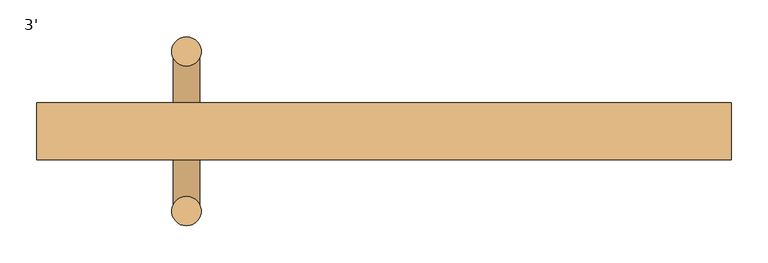
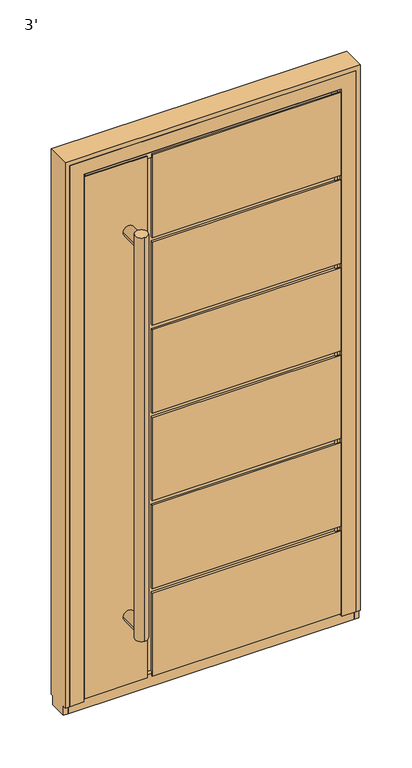
"""IFC4 building model written with IfcOpenShell, lengths in millimetres: door geometry, 3'."""

from ifc_helpers import new_model, si_unit, point, frame, frame_2d, origin, place, context, project, spatial, circle_curve, trimmed, segment, composite_curve, outline, extrude, faceted_brep, source, transform, mapped, element, save


def door_3_44036f4b(model_context):
    return source(origin(), model_context, "Body", "SolidModel", [
        extrude(outline(composite_curve([segment(trimmed(circle_curve(frame_2d((-268.65, 90.8003001)), 20.0), [point((-268.65, 70.8003001))], [point((-268.65, 110.8003001))], False, "CARTESIAN"), True, "CONTINUOUS"), segment(trimmed(circle_curve(frame_2d((-268.65, 90.8003001)), 20.0), [point((-268.65, 110.8003001))], [point((-268.65, 70.8003001))], False, "CARTESIAN"), True, "CONTINUOUS")], self_intersect=False)), frame((0.0, 0.0, 210.0000003), z_axis=(0.0, 0.0, 1.0), x_axis=(1.0, 0.0, 0.0)), (0.0, 0.0, 1.0), 1363.8),
        extrude(outline(composite_curve([segment(trimmed(circle_curve(frame_2d((-268.65, -126.2003001)), 20.0), [point((-268.65, -146.2003001))], [point((-268.65, -106.2003001))], False, "CARTESIAN"), True, "CONTINUOUS"), segment(trimmed(circle_curve(frame_2d((-268.65, -126.2003001)), 20.0), [point((-268.65, -106.2003001))], [point((-268.65, -146.2003001))], False, "CARTESIAN"), True, "CONTINUOUS")], self_intersect=False)), frame((0.0, 0.0, 210.0000003), z_axis=(0.0, 0.0, 1.0), x_axis=(1.0, 0.0, 0.0)), (0.0, 0.0, 1.0), 1363.8),
        extrude(outline(composite_curve([segment(trimmed(circle_curve(frame_2d((241.9000003, -268.65)), 18.0), [point((241.9000003, -286.65))], [point((241.9000003, -250.65))], False, "CARTESIAN"), True, "CONTINUOUS"), segment(trimmed(circle_curve(frame_2d((241.9000003, -268.65)), 18.0), [point((241.9000003, -250.65))], [point((241.9000003, -286.65))], False, "CARTESIAN"), True, "CONTINUOUS")], self_intersect=False)), frame((0.0, -126.2, 0.0), z_axis=(0.0, 1.0, 0.0), x_axis=(0.0, 0.0, 1.0)), (0.0, 0.0, 1.0), 217.0),
        extrude(outline(composite_curve([segment(trimmed(circle_curve(frame_2d((1541.9000003, -268.65)), 18.0), [point((1541.9000003, -286.65))], [point((1541.9000003, -250.65))], False, "CARTESIAN"), True, "CONTINUOUS"), segment(trimmed(circle_curve(frame_2d((1541.9000003, -268.65)), 18.0), [point((1541.9000003, -250.65))], [point((1541.9000003, -286.65))], False, "CARTESIAN"), True, "CONTINUOUS")], self_intersect=False)), frame((0.0, -126.2, 0.0), z_axis=(0.0, 1.0, 0.0), x_axis=(0.0, 0.0, 1.0)), (0.0, 0.0, 1.0), 217.0),
        faceted_brep([(-193.65, 13.8, 306.466667), (383.65, 13.8, 306.466667), (383.65, 13.8, 291.466667), (-193.65, 13.8, 291.466667), (-193.65, 13.8, 35.0), (-208.65, 13.8, 35.0), (-208.65, 13.8, 1748.8000003), (-193.65, 13.8, 1748.8000003), (-193.65, 13.8, 1492.3333337), (383.65, 13.8, 1492.3333337), (383.65, 13.8, 1477.3333337), (-193.65, 13.8, 1477.3333337), (-193.65, 13.8, 1195.866667), (383.65, 13.8, 1195.866667), (383.65, 13.8, 1180.866667), (-193.65, 13.8, 1180.866667), (-193.65, 13.8, 899.4000004), (383.65, 13.8, 899.4000004), (383.65, 13.8, 884.4000004), (-193.65, 13.8, 884.4000004), (-193.65, 13.8, 602.9333337), (383.65, 13.8, 602.9333337), (383.65, 13.8, 587.9333337), (-193.65, 13.8, 587.9333337), (-193.65, 20.8, 587.9333337), (-193.65, 20.8, 306.466667), (383.65, 20.8, 587.9333337), (383.65, 11.7997698, 1748.8000003), (383.65, 11.7997698, 35.0), (383.65, 18.8020472, 35.0), (383.65, 18.8020472, 24.0), (383.65, 20.8, 24.0), (383.65, 20.8, 291.466667), (383.65, 20.8, 306.466667), (383.65, 20.8, 602.9333337), (383.65, 20.8, 884.4000004), (383.65, 20.8, 899.4000004), (383.65, 20.8, 1180.866667), (383.65, 20.8, 1195.866667), (383.65, 20.8, 1477.3333337), (383.65, 20.8, 1492.3333337), (383.65, 20.8, 1748.8000003), (-193.65, 20.8, 602.9333337), (-193.65, 20.8, 884.4000004), (-193.65, 20.8, 899.4000004), (-193.65, 20.8, 1180.866667), (-208.65, 18.8020472, 35.0), (-208.65, 18.8020472, 24.0), (-208.65, 20.8, 24.0), (-208.65, 20.8, 1748.8000003), (-383.65, 11.7997698, 35.0), (-383.65, 18.8020472, 35.0), (-193.65, 18.8020472, 35.0), (-193.65, 20.8, 291.466667), (-193.65, 20.8, 24.0), (-193.65, 18.8020472, 24.0), (-383.65, 18.8020472, 24.0), (-383.65, 20.8, 24.0), (-383.65, 20.8, 1748.8000003), (-193.65, 20.8, 1195.866667), (-193.65, 20.8, 1477.3333337), (-193.65, 20.8, 1492.3333337), (-193.65, 20.8, 1748.8000003), (408.65, -56.2, 10.0000003), (-193.65, -56.2, 10.0000003), (-193.65, -53.2, 10.0000003), (408.65, -53.2, 10.0000003), (-408.65, -53.2, 10.0000003), (-208.65, -53.2, 10.0000003), (-208.65, -56.2, 10.0000003), (-408.65, -56.2, 10.0000003), (408.65, -56.2, 306.466667), (408.65, -53.2, 306.466667), (408.65, -53.2, 587.9333337), (408.65, -56.2, 587.9333337), (408.65, -56.2, 899.4000004), (408.65, -53.2, 899.4000004), (408.65, -53.2, 1180.866667), (408.65, -56.2, 1180.866667), (408.65, -56.2, 602.9333337), (408.65, -53.2, 602.9333337), (408.65, -53.2, 884.4000004), (408.65, -56.2, 884.4000004), (408.65, -56.2, 1195.866667), (408.65, -53.2, 1195.866667), (408.65, -53.2, 1477.3333337), (408.65, -56.2, 1477.3333337), (408.65, -56.2, 1773.8000003), (408.65, -56.2, 1492.3333337), (408.65, -53.2, 1492.3333337), (408.65, -53.2, 1773.8000003), (408.65, -53.2, 291.466667), (408.65, -56.2, 291.466667), (-193.65, -53.2, 25.5), (393.15, -53.2, 25.5), (393.15, -53.2, 291.466667), (393.15, -53.2, 306.466667), (393.15, -53.2, 587.9333337), (393.15, -53.2, 899.4000004), (393.15, -53.2, 1180.866667), (393.15, -53.2, 602.9333337), (393.15, -53.2, 884.4000004), (-393.15, -53.2, 25.5), (-208.65, -53.2, 25.5), (-408.65, -53.2, 1773.8000003), (-208.65, -53.2, 1773.8000003), (-208.65, -53.2, 1758.3000003), (-393.15, -53.2, 1758.3000003), (393.15, -53.2, 1195.866667), (393.15, -53.2, 1477.3333337), (393.15, -53.2, 1492.3333337), (393.15, -53.2, 1758.3000003), (-193.65, -53.2, 1758.3000003), (-193.65, -53.2, 1773.8000003), (-193.65, -49.2, 291.466667), (-193.65, -49.2, 25.5), (-193.65, -56.2, 291.466667), (-208.65, -56.2, 1773.8000003), (-408.65, -56.2, 1773.8000003), (-193.65, -56.2, 587.9333337), (-193.65, -56.2, 306.466667), (-193.65, -56.2, 1180.866667), (-193.65, -56.2, 899.4000004), (-193.65, -56.2, 884.4000004), (-193.65, -56.2, 602.9333337), (-193.65, -56.2, 1477.3333337), (-193.65, -56.2, 1195.866667), (-193.65, -56.2, 1773.8000003), (-193.65, -56.2, 1492.3333337), (-208.65, -49.2, 1758.3000003), (-208.65, -49.2, 25.5), (-383.65, 11.7997698, 1748.8000003), (393.15, 11.7997698, 1758.3000003), (393.15, 11.7997698, 25.5), (-393.15, 11.7997698, 25.5), (-393.15, 11.7997698, 1758.3000003), (393.15, -49.2, 1492.3333337), (393.15, -49.2, 1477.3333337), (393.15, -49.2, 1195.866667), (393.15, -49.2, 1180.866667), (393.15, -49.2, 899.4000004), (393.15, -49.2, 884.4000004), (393.15, -49.2, 602.9333337), (393.15, -49.2, 587.9333337), (393.15, -49.2, 306.466667), (393.15, -49.2, 291.466667), (-193.65, -49.2, 1477.3333337), (-193.65, -49.2, 1492.3333337), (-193.65, -49.2, 1758.3000003), (-193.65, -49.2, 306.466667), (-193.65, -49.2, 587.9333337), (-193.65, -49.2, 602.9333337), (-193.65, -49.2, 884.4000004), (-193.65, -49.2, 899.4000004), (-193.65, -49.2, 1180.866667), (-193.65, -49.2, 1195.866667)], [[[0, 1, 2, 3, 4, 5, 6, 7, 8, 9, 10, 11, 12, 13, 14, 15, 16, 17, 18, 19, 20, 21, 22, 23]], [[23, 24, 25, 0]], [[23, 22, 26, 24]], [[27, 28, 29, 30, 31, 32, 2, 1, 33, 26, 22, 21, 34, 35, 18, 17, 36, 37, 14, 13, 38, 39, 10, 9, 40, 41]], [[42, 34, 21, 20]], [[19, 43, 42, 20]], [[19, 18, 35, 43]], [[44, 36, 17, 16]], [[15, 45, 44, 16]], [[5, 46, 47, 48, 49, 6]], [[28, 50, 51, 46, 5, 4, 52, 29]], [[53, 54, 55, 52, 4, 3]], [[3, 2, 32, 53]], [[25, 33, 1, 0]], [[29, 52, 55, 30]], [[56, 47, 46, 51]], [[30, 55, 54, 31]], [[57, 48, 47, 56]], [[36, 44, 45, 37]], [[34, 42, 43, 35]], [[33, 25, 24, 26]], [[54, 53, 32, 31]], [[58, 49, 48, 57]], [[38, 59, 60, 39]], [[41, 40, 61, 62]], [[63, 64, 65, 66]], [[67, 68, 69, 70]], [[71, 72, 73, 74]], [[75, 76, 77, 78]], [[79, 80, 81, 82]], [[83, 84, 85, 86]], [[87, 88, 89, 90]], [[66, 91, 92, 63]], [[65, 93, 94, 95, 91, 66]], [[72, 96, 97, 73]], [[76, 98, 99, 77]], [[80, 100, 101, 81]], [[102, 103, 68, 67, 104, 105, 106, 107]], [[84, 108, 109, 85]], [[90, 89, 110, 111, 112, 113]], [[114, 115, 93, 65, 64, 116]], [[70, 69, 117, 118]], [[63, 92, 116, 64]], [[74, 119, 120, 71]], [[78, 121, 122, 75]], [[82, 123, 124, 79]], [[86, 125, 126, 83]], [[87, 127, 128, 88]], [[70, 118, 104, 67]], [[129, 106, 105, 117, 69, 68, 103, 130]], [[58, 57, 56, 51, 50, 131]], [[132, 133, 134, 135], [131, 50, 28, 27]], [[111, 110, 136, 137, 109, 108, 138, 139, 99, 98, 140, 141, 101, 100, 142, 143, 97, 96, 144, 145, 95, 94, 133, 132]], [[94, 93, 115, 130, 103, 102, 134, 133]], [[135, 134, 102, 107]], [[146, 137, 136, 147, 148, 129, 130, 115, 114, 145, 144, 149, 150, 143, 142, 151, 152, 141, 140, 153, 154, 139, 138, 155]], [[153, 122, 121, 154]], [[153, 140, 98, 76, 75, 122]], [[123, 82, 81, 101, 141, 152]], [[151, 124, 123, 152]], [[151, 142, 100, 80, 79, 124]], [[119, 74, 73, 97, 143, 150]], [[149, 120, 119, 150]], [[149, 144, 96, 72, 71, 120]], [[116, 92, 91, 95, 145, 114]], [[15, 14, 37, 45]], [[59, 38, 13, 12]], [[11, 60, 59, 12]], [[11, 10, 39, 60]], [[61, 40, 9, 8]], [[8, 7, 62, 61]], [[125, 86, 85, 109, 137, 146]], [[128, 127, 113, 112, 148, 147]], [[121, 78, 77, 99, 139, 154]], [[155, 138, 108, 84, 83, 126]], [[155, 126, 125, 146]], [[147, 136, 110, 89, 88, 128]], [[90, 113, 127, 87]], [[118, 117, 105, 104]], [[132, 135, 107, 106, 129, 148, 112, 111]], [[27, 41, 62, 7, 6, 49, 58, 131]]]),
        faceted_brep([(-457.2, -56.2, 0.0), (-457.2, -47.1997571, 0.0), (-412.7, -47.1997571, 0.0), (-412.7, -56.2, 0.0), (-403.2, 16.2999958, 0.0), (-403.2, 11.8, 0.0), (-457.2, 11.8, 0.0), (-457.2, 20.8, 0.0), (-387.7, 20.8, 0.0), (-387.7, 16.2999958, 0.0), (457.2, 20.8, 0.0), (457.2, 11.8, 0.0), (403.2, 11.8, 0.0), (403.2, 16.2999958, 0.0), (387.7, 16.2999958, 0.0), (387.7, 20.8, 0.0), (412.7, -47.1997571, 0.0), (457.2, -47.1997571, 0.0), (457.2, -56.2, 0.0), (412.7, -56.2, 0.0), (-457.2, 11.8, -30.0), (-457.2, -47.1997571, -30.0), (-457.2, -56.2, 1828.8), (-457.2, 20.8, 1828.8), (-412.7, -56.2, 1784.3), (412.7, -56.2, 1784.3), (457.2, -56.2, 1828.8), (457.2, 20.8, 1828.8), (457.2, -47.1997571, -30.0), (457.2, 11.8, -30.0), (387.7, 20.8, 1759.3), (-387.7, 20.8, 1759.3), (-403.2, -47.2, 1774.8), (-403.2, -47.2, 14.5), (-403.2, 11.8, 14.5), (-403.2, 16.2999958, 1774.8), (403.2, 16.2999958, 1774.8), (403.2, -47.2, 1774.8), (403.2, 11.8, 14.5), (403.2, -47.2, 14.5), (-412.7, -47.2, 1784.3), (412.7, -47.2, 1784.3), (-387.7, 16.2999958, 1759.3), (387.7, 16.2999958, 1759.3)], [[[0, 1, 2, 3]], [[4, 5, 6, 7, 8, 9]], [[10, 11, 12, 13, 14, 15]], [[16, 17, 18, 19]], [[7, 6, 20, 21, 1, 0, 22, 23]], [[3, 24, 25, 19, 18, 26, 22, 0]], [[22, 26, 27, 23]], [[18, 17, 28, 29, 11, 10, 27, 26]], [[7, 23, 27, 10, 15, 30, 31, 8]], [[32, 33, 34, 5, 4, 35]], [[35, 36, 37, 32]], [[36, 13, 12, 38, 39, 37]], [[40, 24, 3, 2]], [[16, 41, 40, 2, 1, 21, 28, 17], [37, 39, 33, 32]], [[9, 42, 43, 14, 13, 36, 35, 4]], [[8, 31, 42, 9]], [[24, 40, 41, 25]], [[30, 43, 42, 31]], [[19, 25, 41, 16]], [[14, 43, 30, 15]], [[20, 6, 5, 34, 38, 12, 11, 29]], [[39, 38, 34, 33]], [[20, 29, 28, 21]]]),
        faceted_brep([(-457.2, -47.2, -30.0), (-472.2, -47.2, -30.0), (-472.2, 11.8, -30.0), (-457.2, 11.8, -30.0), (-457.2, -56.2, 1828.8), (-457.2, -56.2, 0.0), (-457.2, -47.2, 0.0), (-457.2, 11.8, 0.0), (-457.2, 20.8, 0.0), (-457.2, 20.8, 1828.8), (-472.2, 11.8, 0.0), (472.2, 11.8, 0.0), (472.2, 11.8, -30.0), (457.2, 11.8, -30.0), (457.2, 11.8, 0.0), (-472.2, 20.8, 1843.8), (-472.2, 20.8, 0.0), (-472.2, -47.2, 0.0), (-472.2, -56.2, 0.0), (-472.2, -56.2, 1843.8), (457.2, -47.2, 0.0), (457.2, -47.2, -30.0), (472.2, -47.2, -30.0), (472.2, -47.2, 0.0), (457.2, 20.8, 1828.8), (457.2, 20.8, 0.0), (457.2, -56.2, 0.0), (457.2, -56.2, 1828.8), (472.2, -56.2, 0.0), (472.2, -56.2, 1843.8), (472.2, 20.8, 0.0), (472.2, 20.8, 1843.8)], [[[0, 1, 2, 3]], [[4, 5, 6, 0, 3, 7, 8, 9]], [[7, 3, 2, 10]], [[11, 12, 13, 14]], [[15, 16, 10, 2, 1, 17, 18, 19]], [[17, 1, 0, 6]], [[20, 21, 22, 23]], [[24, 25, 14, 13, 21, 20, 26, 27]], [[27, 26, 28, 29, 19, 18, 5, 4]], [[6, 5, 18, 17]], [[23, 28, 26, 20]], [[22, 21, 13, 12]], [[10, 16, 8, 7]], [[14, 25, 30, 11]], [[9, 8, 16, 15, 31, 30, 25, 24]], [[29, 28, 23, 22, 12, 11, 30, 31]], [[9, 24, 27, 4]], [[19, 29, 31, 15]]]),
    ])


if __name__ == "__main__":
    model = new_model("IFC4")
    model_context = context("Model", 3, world=origin())
    ifc_project = project(units=[si_unit("LENGTHUNIT", "METRE", prefix="MILLI")], contexts=[model_context])
    site = spatial("IfcSite", under=ifc_project)
    building = spatial("IfcBuilding", under=site)
    placement = place(None, origin())
    door_3_shape = door_3_44036f4b(model_context)
    element("IfcDoor", 1, ObjectType="3'", at=placement, inside=building, context=model_context, shape_type="MappedRepresentation", body=[
        mapped(door_3_shape, transform((0.0, 0.0, 0.0), x_axis=(1.0, 0.0, 0.0), y_axis=(0.0, 1.0, 0.0), z_axis=(0.0, 0.0, 1.0))),
    ])
    save(model, "model.ifc")

# Revit data of these elements
# Type "3'"
#   Type Mark = "41"
#   Water resistance = "up to Class E900, EN 12208:2001"
#   Uniclass2015Version = "v1.21"
#   Uniclass2015Reference = "Ss_25_30_20_30"
#   Uniclass2015Description = "Frame and door leaf system"
#   URL = "www.aluprof.com"
#   Type IFC Predefined Type = "USERDEFINED"
#   Right-hand / Left-hand door [instance default] = ""
#   Resistance to wind load = "up to Class C5/B5, EN 12210:2001"
#   Insert type = "ST"
#   Hardware [instance default] = ""
#   Product page = "https://aluprof.com/en/architects/offer/window-and-door-systems/panel-doors#visualisation"
#   Operation = "SinglePanelOutwardOpening"
#   Opening type = "Outward"
#   NBSReference = "25-50-20/125"
#   NBSDescription = "Frame and door leaf system"
#   Important = "The actual acceptable construction dimensions are dependent on the selection of profiles and hardware, glazing type, construction weight and the construction’s operating conditions. These should be determined by a suitably qualified person, and using ALUPROF’s calculation software"
#   IfcExportType = "USERDEFINED"
#   IfcExportAs = "IfcDoorType"
#   Handle type [instance default] = ""
#   Manufacturer = "ALUPROF SA"
#   Export Type to IFC As = "IfcDoorType"
#   Door sill type [instance default] = ""
#   Description = "External single-leaf panel door outward opening"
#   Model = "MB-86 ST Panel Door AD07"
#   Content of the recyclate in the material = "69.2%"
#   COBie.Type.WarrantyDurationParts = ""
#   COBie.Type.Name = ""
#   COBie.Type.Manufacturer = "ALUPROF SA"
#   COBie.Space.Name = ""
#   COBie.Floor.Name = ""
#   COBie.Facility.Name = ""
#   COBie.CreatedOn = ""
#   COBie.Component.WarrantyStartDate = ""
#   COBie.Component.Name = "MB-86 ST Panel Door AD07"
#   Burglar resistance = "RC2"
#   Air permeability = "up to Class 4, EN 12207:2001"
#   Width of the active leaf = 2' - 8.17717"
#   Placement in wall = 0' - 0.7874"
#   Thickness = 0' - 3.0315"
#   Height of the opening sash = 5' - 9.44094"
#   Handle Offset = 3' - 5.33858"
#   Rough Height = 6' - 2.40945"
#   Rough Width = 3' - 1.1811"
#   Height = 6' - 0"
#   Width = 3' - 0"
#   Construction depth = 0' - 3.0315"
#   Clear opening width = 2' - 3.94882"
#   Clear opening height = 5' - 8.47638"
#   Height of the array = 0' - 11.08136"
#   Schedule No. [instance default] = 1
#   Handrail [instance default] = yes
#   IsExternal = yes
#   Handle [instance default] = no
#   Door closer [instance default] = no
#   Function = 1
#   COBie.Type = yes
#   COBie = yes
#   Access control [instance default] = no
#   Panel = element 371215
#   Wall Closure = (empty or 0)
